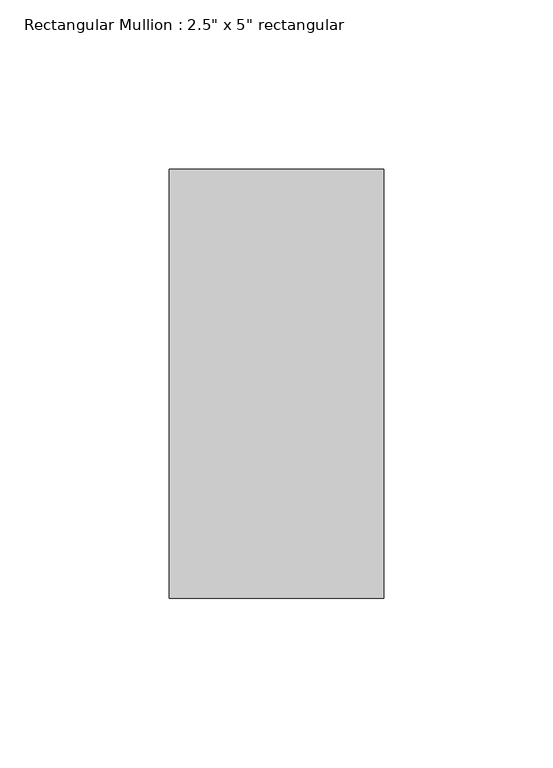
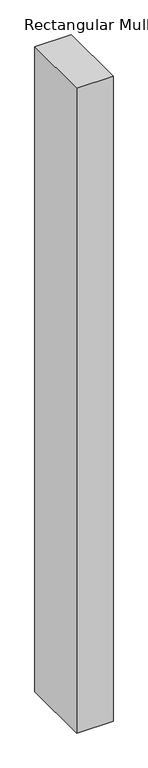
"""IFC4 building model written with IfcOpenShell, lengths in millimetres: member geometry."""

from ifc_helpers import new_model, si_unit, frame, origin, place, context, project, spatial, polyline, outline, extrude, source, transform, mapped, element, save


def member_2d647432(model_context):
    return source(origin(), model_context, "Body", "SweptSolid", [
        extrude(outline(polyline([(31.75, 63.5), (31.75, -63.5), (-31.75, -63.5), (-31.75, 63.5), (31.75, 63.5)])), frame((0.0, 0.0, -1193.8), z_axis=(0.0, 0.0, 1.0), x_axis=(1.0, 0.0, 0.0)), (0.0, 0.0, 1.0), 1193.8),
    ])


if __name__ == "__main__":
    model = new_model("IFC4")
    model_context = context("Model", 3, world=origin())
    ifc_project = project(units=[si_unit("LENGTHUNIT", "METRE", prefix="MILLI")], contexts=[model_context])
    site = spatial("IfcSite", under=ifc_project)
    building = spatial("IfcBuilding", under=site)
    placement = place(None, origin())
    member_shape = member_2d647432(model_context)
    element("IfcMember", 1, ObjectType="Rectangular Mullion : 2.5\" x 5\" rectangular", at=placement, inside=building, context=model_context, shape_type="MappedRepresentation", body=[
        mapped(member_shape, transform((0.0, 0.0, 0.0), x_axis=(1.0, 0.0, 0.0), y_axis=(0.0, 1.0, 0.0), z_axis=(0.0, 0.0, 1.0))),
    ])
    save(model, "model.ifc")

# Revit data of these elements
# Type "Rectangular Mullion : 2.5\" x 5\" rectangular"
#   built-in parameter 1007304 = 0.416667 (stored number, unit not read)
#   built-in parameter 1007301 = 0.104167 (stored number, unit not read)
#   built-in parameter 1007300 = 0.104167 (stored number, unit not read)
